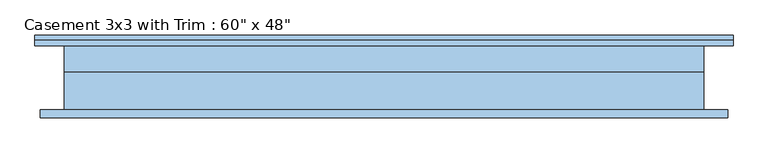
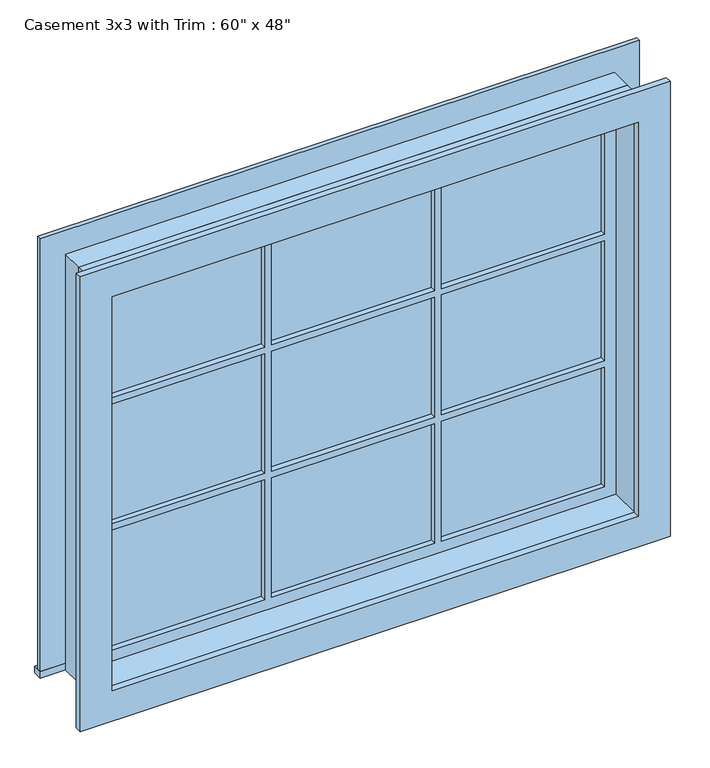
"""IFC4 building model written with IfcOpenShell, lengths in millimetres: window geometry."""

from ifc_helpers import new_model, si_unit, frame, origin, place, context, project, spatial, polyline, outline, extrude, source, transform, mapped, element, save


def window_1f50baaf(model_context):
    return source(origin(), model_context, "Body", "SweptSolid", [
        extrude(outline(polyline([(-831.85, 101.6), (831.85, 101.6), (831.85, 76.2), (-831.85, 76.2), (-831.85, 101.6)])), frame((0.0, 0.0, 914.4), z_axis=(0.0, 0.0, 1.0), x_axis=(1.0, 0.0, 0.0)), (0.0, 0.0, 1.0), 19.05),
        extrude(outline(polyline([(2114.55, -742.95), (2114.55, 742.95), (933.45, 742.95), (933.45, 831.85), (2203.45, 831.85), (2203.45, -831.85), (933.45, -831.85), (933.45, -742.95), (2114.55, -742.95)])), frame((0.0, 76.2, 0.0), z_axis=(0.0, 1.0, 0.0), x_axis=(0.0, 0.0, 1.0)), (0.0, 0.0, 1.0), 12.7),
        extrude(outline(polyline([(245.5333333, 41.275), (698.5, 41.275), (698.5, 28.575), (245.5333333, 28.575), (245.5333333, 41.275)])), frame((0.0, 0.0, 1718.7333333), z_axis=(0.0, 0.0, 1.0), x_axis=(1.0, 0.0, 0.0)), (0.0, 0.0, 1.0), 351.3666667),
        extrude(outline(polyline([(-226.4833333, 41.275), (226.4833333, 41.275), (226.4833333, 28.575), (-226.4833333, 28.575), (-226.4833333, 41.275)])), frame((0.0, 0.0, 1718.7333333), z_axis=(0.0, 0.0, 1.0), x_axis=(1.0, 0.0, 0.0)), (0.0, 0.0, 1.0), 351.3666667),
        extrude(outline(polyline([(-698.5, 41.275), (-245.5333333, 41.275), (-245.5333333, 28.575), (-698.5, 28.575), (-698.5, 41.275)])), frame((0.0, 0.0, 1718.7333333), z_axis=(0.0, 0.0, 1.0), x_axis=(1.0, 0.0, 0.0)), (0.0, 0.0, 1.0), 351.3666667),
        extrude(outline(polyline([(-698.5, 41.275), (-245.5333333, 41.275), (-245.5333333, 28.575), (-698.5, 28.575), (-698.5, 41.275)])), frame((0.0, 0.0, 1348.3166667), z_axis=(0.0, 0.0, 1.0), x_axis=(1.0, 0.0, 0.0)), (0.0, 0.0, 1.0), 351.3666667),
        extrude(outline(polyline([(-226.4833333, 41.275), (226.4833333, 41.275), (226.4833333, 28.575), (-226.4833333, 28.575), (-226.4833333, 41.275)])), frame((0.0, 0.0, 1348.3166667), z_axis=(0.0, 0.0, 1.0), x_axis=(1.0, 0.0, 0.0)), (0.0, 0.0, 1.0), 351.3666667),
        extrude(outline(polyline([(245.5333333, 41.275), (698.5, 41.275), (698.5, 28.575), (245.5333333, 28.575), (245.5333333, 41.275)])), frame((0.0, 0.0, 1348.3166667), z_axis=(0.0, 0.0, 1.0), x_axis=(1.0, 0.0, 0.0)), (0.0, 0.0, 1.0), 351.3666667),
        extrude(outline(polyline([(245.5333333, 41.275), (698.5, 41.275), (698.5, 28.575), (245.5333333, 28.575), (245.5333333, 41.275)])), frame((0.0, 0.0, 977.9), z_axis=(0.0, 0.0, 1.0), x_axis=(1.0, 0.0, 0.0)), (0.0, 0.0, 1.0), 351.3666667),
        extrude(outline(polyline([(-226.4833333, 41.275), (226.4833333, 41.275), (226.4833333, 28.575), (-226.4833333, 28.575), (-226.4833333, 41.275)])), frame((0.0, 0.0, 977.9), z_axis=(0.0, 0.0, 1.0), x_axis=(1.0, 0.0, 0.0)), (0.0, 0.0, 1.0), 351.3666667),
        extrude(outline(polyline([(-698.5, 41.275), (-245.5333333, 41.275), (-245.5333333, 28.575), (-698.5, 28.575), (-698.5, 41.275)])), frame((0.0, 0.0, 977.9), z_axis=(0.0, 0.0, 1.0), x_axis=(1.0, 0.0, 0.0)), (0.0, 0.0, 1.0), 351.3666667),
        extrude(outline(polyline([(2190.75, 819.15), (2190.75, -819.15), (857.25, -819.15), (857.25, 819.15), (2190.75, 819.15)]), holes=[polyline([(2101.85, 730.25), (946.15, 730.25), (946.15, -730.25), (2101.85, -730.25), (2101.85, 730.25)])]), frame((0.0, -95.25, 0.0), z_axis=(0.0, 1.0, 0.0), x_axis=(0.0, 0.0, 1.0)), (0.0, 0.0, 1.0), 19.05),
        extrude(outline(polyline([(2114.55, -742.95), (933.45, -742.95), (933.45, 742.95), (2114.55, 742.95), (2114.55, -742.95)]), holes=[polyline([(2070.1, -245.5333333), (1718.7333333, -245.5333333), (1718.7333333, -698.5), (2070.1, -698.5), (2070.1, -245.5333333)]), polyline([(1699.6833333, -245.5333333), (1348.3166667, -245.5333333), (1348.3166667, -698.5), (1699.6833333, -698.5), (1699.6833333, -245.5333333)]), polyline([(1329.2666667, -245.5333333), (977.9, -245.5333333), (977.9, -698.5), (1329.2666667, -698.5), (1329.2666667, -245.5333333)]), polyline([(2070.1, 226.4833333), (1718.7333333, 226.4833333), (1718.7333333, -226.4833333), (2070.1, -226.4833333), (2070.1, 226.4833333)]), polyline([(1699.6833333, 226.4833333), (1348.3166667, 226.4833333), (1348.3166667, -226.4833333), (1699.6833333, -226.4833333), (1699.6833333, 226.4833333)]), polyline([(1329.2666667, 226.4833333), (977.9, 226.4833333), (977.9, -226.4833333), (1329.2666667, -226.4833333), (1329.2666667, 226.4833333)]), polyline([(2070.1, 698.5), (1718.7333333, 698.5), (1718.7333333, 245.5333333), (2070.1, 245.5333333), (2070.1, 698.5)]), polyline([(1699.6833333, 698.5), (1348.3166667, 698.5), (1348.3166667, 245.5333333), (1699.6833333, 245.5333333), (1699.6833333, 698.5)]), polyline([(1329.2666667, 698.5), (977.9, 698.5), (977.9, 245.5333333), (1329.2666667, 245.5333333), (1329.2666667, 698.5)])]), frame((0.0, 12.7, 0.0), z_axis=(0.0, 1.0, 0.0), x_axis=(0.0, 0.0, 1.0)), (0.0, 0.0, 1.0), 44.45),
        extrude(outline(polyline([(2133.6, -762.0), (914.4, -762.0), (914.4, 762.0), (2133.6, 762.0), (2133.6, -762.0)]), holes=[polyline([(2101.85, -730.25), (2101.85, 730.25), (946.15, 730.25), (946.15, -730.25), (2101.85, -730.25)])]), frame((0.0, -76.2, 0.0), z_axis=(0.0, 1.0, 0.0), x_axis=(0.0, 0.0, 1.0)), (0.0, 0.0, 1.0), 88.9),
        extrude(outline(polyline([(2133.6, 762.0), (2133.6, -762.0), (914.4, -762.0), (914.4, 762.0), (2133.6, 762.0)]), holes=[polyline([(2114.55, 742.95), (933.45, 742.95), (933.45, -742.95), (2114.55, -742.95), (2114.55, 742.95)])]), frame((0.0, 12.7, 0.0), z_axis=(0.0, 1.0, 0.0), x_axis=(0.0, 0.0, 1.0)), (0.0, 0.0, 1.0), 63.5),
    ])


if __name__ == "__main__":
    model = new_model("IFC4")
    model_context = context("Model", 3, world=origin())
    ifc_project = project(units=[si_unit("LENGTHUNIT", "METRE", prefix="MILLI")], contexts=[model_context])
    site = spatial("IfcSite", under=ifc_project)
    building = spatial("IfcBuilding", under=site)
    placement = place(None, origin())
    window_shape = window_1f50baaf(model_context)
    element("IfcWindow", 1, ObjectType="Casement 3x3 with Trim : 60\" x 48\"", at=placement, inside=building, context=model_context, shape_type="MappedRepresentation", body=[
        mapped(window_shape, transform((0.0, 0.0, 0.0), x_axis=(1.0, 0.0, 0.0), y_axis=(0.0, 1.0, 0.0), z_axis=(0.0, 0.0, 1.0))),
    ])
    save(model, "model.ifc")

# Revit data of these elements
# Type "Casement 3x3 with Trim : 60\" x 48\""
#   Type Mark = "10"
#   Construction Type Id = "GSP4R"
#   Assembly Code = "B2020100"
#   Analytic Construction = "1/8 in Pilkington single glazing"
#   Visual Light Transmittance = 0.9
#   Solar Heat Gain Coefficient = 0.78
#   Heat Transfer Coefficient (U) = 0.6496 BTU/(h·ft²·°F)
#   Height = 4' - 0"
#   Default Sill Height = 3' - 0"
#   Trim Projection - Ext. = 0' - 0 1/2"
#   Trim Projection - Int. = 0' - 0 3/4"
#   Trim Width - Exterior = 0' - 3 1/2"
#   Trim Width - Interior = 0' - 3 1/2"
#   Width = 5' - 0"
#   Window Inset = 0' - 0 3/4"
#   Define Thermal Properties by = 1
#   Glass Pane Material = Glass
#   Sash Material = Sash
#   Trim Exterior Material = Trim
#   Trim Interior Material = Trim
#   Wall Closure = (empty or 0)
# Element 1 (IfcWindow, "Casement 3x3 with Trim : 60\" x 48\"")
#   Materials on its faces: "Sash", "Glass", "Trim"
# Materials
#   "Glass": class "Glass", colour RGB 0 128 192, transparency 0.75, Description = "Soda Lime Glass", Cost = 0
#   "Sash": class "Wood", colour RGB 224 178 126, transparency 0
#   "Trim": class "Wood", colour RGB 224 178 126, transparency 0
